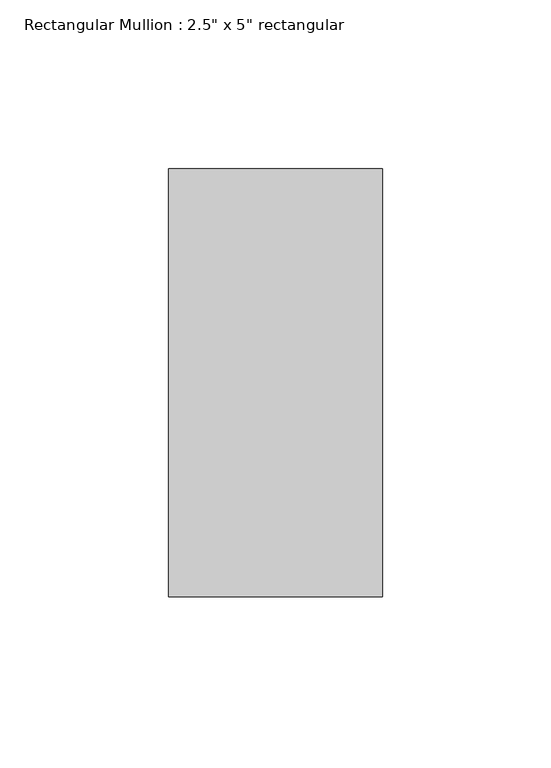
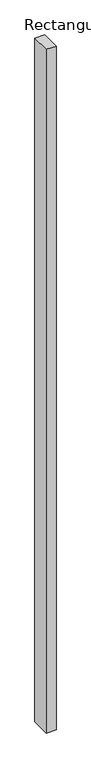
"""IFC4 building model written with IfcOpenShell, lengths in millimetres: member geometry."""

from ifc_helpers import new_model, si_unit, frame, origin, place, context, project, spatial, polyline, outline, extrude, source, transform, mapped, element, save


def member_61d9bab4(model_context):
    return source(origin(), model_context, "Body", "SweptSolid", [
        extrude(outline(polyline([(0.0, 63.5), (0.0, -63.5), (-63.5, -63.5), (-63.5, 63.5), (0.0, 63.5)])), frame((0.0, 0.0, -4679.95), z_axis=(0.0, 0.0, 1.0), x_axis=(1.0, 0.0, 0.0)), (0.0, 0.0, 1.0), 4679.95),
    ])


if __name__ == "__main__":
    model = new_model("IFC4")
    model_context = context("Model", 3, world=origin())
    ifc_project = project(units=[si_unit("LENGTHUNIT", "METRE", prefix="MILLI")], contexts=[model_context])
    site = spatial("IfcSite", under=ifc_project)
    building = spatial("IfcBuilding", under=site)
    placement = place(None, origin())
    member_shape = member_61d9bab4(model_context)
    element("IfcMember", 1, ObjectType="Rectangular Mullion : 2.5\" x 5\" rectangular", at=placement, inside=building, context=model_context, shape_type="MappedRepresentation", body=[
        mapped(member_shape, transform((0.0, 0.0, 0.0), x_axis=(1.0, 0.0, 0.0), y_axis=(0.0, 1.0, 0.0), z_axis=(0.0, 0.0, 1.0))),
    ])
    save(model, "model.ifc")

# Revit data of these elements
# Type "Rectangular Mullion : 2.5\" x 5\" rectangular"
#   built-in parameter 1007304 = 0.416667 (stored number, unit not read)
#   built-in parameter 1007301 = 0.104167 (stored number, unit not read)
#   built-in parameter 1007300 = 0.104167 (stored number, unit not read)
# Element 1 (IfcMember, "Rectangular Mullion : 2.5\" x 5\" rectangular")
#   Materials on its faces: "Aluminum"
# Materials
#   "Aluminum": class "Metal", colour RGB 247 247 247, transparency 0, Description = "Aluminum 6061", Cost = 0
